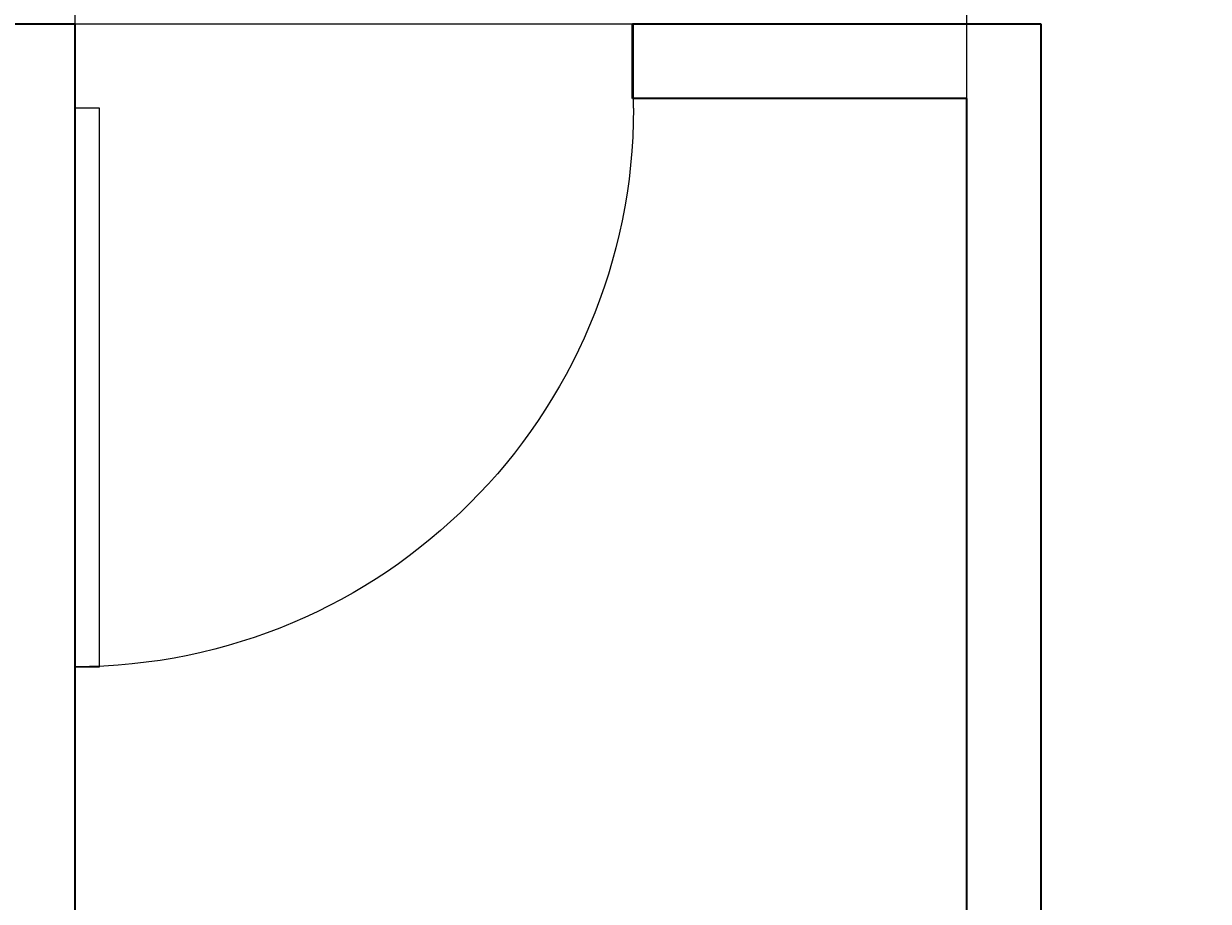
# Model space of a CAD drawing. Units: feet. Extents: x 105 to 1094, y -88 to 588.
# Tile 20 of 59: x 372 to 436, y 307 to 354. Entities that reach past the tile are written whole.
import ezdxf

# ---------------------------------------------------------------- set-up
doc = ezdxf.new("R2010")
doc.units = ezdxf.units.FT
doc.header["$MEASUREMENT"] = 0
for name, color, linetype, lineweight in [('A-ANNO-DIMS', 2, 'Continuous', 18), ('A-DOOR', 3, 'Continuous', 25), ('A-WALL', 7, 'Continuous', 35)]:
    doc.layers.add(name, color=color, linetype=linetype, lineweight=lineweight)
doc.styles.get("Standard").update_dxf_attribs({"font": 'arial.ttf'})
doc.dimstyles.get("Standard").update_dxf_attribs({"dimtxt": 0.18, "dimasz": 0.18, "dimexe": 0.18, "dimexo": 0.0625, "dimgap": 0.09, "dimtad": 0, "dimtih": 1, "dimtoh": 1, "dimdec": 4, "dimzin": 0, "dimdsep": 46, "dimtxsty": 'Standard', "dimcen": 0.09, "dimadec": 0, "dimazin": 0, "dimtfac": 1, "dimtdec": 4, "dimtofl": 0, "dimtmove": 0, "dimatfit": 3, "dimfxl": 1, "dimtolj": 1, "dimtzin": 0, "dimarcsym": 0})

# ---------------------------------------------------------------- blocks, each defined once
blk = doc.blocks.new('*U2')
for p, q in [((0, 0), (0, -6)), ((40, 0), (40, -6))]:
    blk.add_line(p, q)
blk.add_lwpolyline([(0, 0), (0, 40), (1.75, 40), (1.75, 0)], close=True)
blk.add_arc((0, 0), 40, 0, 90)
blk = doc.blocks.new('*D21')
at = {"layer": 'A-ANNO-DIMS', "color": 0, "lineweight": -2, "transparency": 16777216}
for p, q in [((849.626, 543.081), (105.458, 543.081)), ((105.638, 542.901), (105.638, 250.263)), ((105.638, -42.739), (105.638, 249.899)), ((849.626, -42.919), (105.458, -42.919))]:
    blk.add_line(p, q, dxfattribs=at)
at = {"layer": 'A-ANNO-DIMS', "color": 0, "transparency": 16777216}
for points in [[(105.608, 542.901), (105.668, 542.901), (105.638, 543.081)], [(105.608, -42.739), (105.668, -42.739), (105.638, -42.919)]]:
    blk.add_solid(points, dxfattribs=at)
at = {"layer": 'Defpoints', "color": 0, "transparency": 16777216}
for p in [(105.638, 543.081), (849.688, 543.081), (849.688, -42.919)]:
    blk.add_point(p, dxfattribs=at)
at = {"layer": 'A-ANNO-DIMS', "color": 0, "transparency": 16777216, "insert": (105.638, 250.081), "char_height": 0.18, "attachment_point": 5}
blk.add_mtext('\\A1;586', dxfattribs=at)
blk = doc.blocks.new('*D33')
at = {"layer": 'A-ANNO-DIMS', "color": 0, "lineweight": -2, "transparency": 16777216}
for p, q in [((646.626, 395.081), (105.458, 395.081)), ((105.638, 394.901), (105.638, 345.263)), ((105.638, 295.261), (105.638, 344.899)), ((646.626, 295.081), (105.458, 295.081))]:
    blk.add_line(p, q, dxfattribs=at)
at = {"layer": 'A-ANNO-DIMS', "color": 0, "transparency": 16777216}
for points in [[(105.608, 394.901), (105.668, 394.901), (105.638, 395.081)], [(105.608, 295.261), (105.668, 295.261), (105.638, 295.081)]]:
    blk.add_solid(points, dxfattribs=at)
at = {"layer": 'Defpoints', "color": 0, "transparency": 16777216}
for p in [(646.688, 395.081), (105.638, 295.081), (646.688, 295.081)]:
    blk.add_point(p, dxfattribs=at)
at = {"layer": 'A-ANNO-DIMS', "color": 0, "transparency": 16777216, "insert": (105.638, 345.081), "char_height": 0.18, "attachment_point": 5}
blk.add_mtext('\\A1;100', dxfattribs=at)
blk = doc.blocks.new('*D51')
at = {"layer": 'A-ANNO-DIMS', "color": 0, "lineweight": -2, "transparency": 16777216}
for p, q in [((432.626, 394.081), (105.458, 394.081)), ((105.638, 393.901), (105.638, 374.263)), ((105.638, 354.261), (105.638, 373.899)), ((426.626, 354.081), (105.458, 354.081))]:
    blk.add_line(p, q, dxfattribs=at)
at = {"layer": 'A-ANNO-DIMS', "color": 0, "transparency": 16777216}
for points in [[(105.608, 393.901), (105.668, 393.901), (105.638, 394.081)], [(105.608, 354.261), (105.668, 354.261), (105.638, 354.081)]]:
    blk.add_solid(points, dxfattribs=at)
at = {"layer": 'Defpoints', "color": 0, "transparency": 16777216}
for p in [(432.688, 394.081), (105.638, 354.081), (426.688, 354.081)]:
    blk.add_point(p, dxfattribs=at)
at = {"layer": 'A-ANNO-DIMS', "color": 0, "transparency": 16777216, "insert": (105.638, 374.081), "char_height": 0.18, "attachment_point": 5}
blk.add_mtext('\\A1;40', dxfattribs=at)
blk = doc.blocks.new('*D56')
at = {"layer": 'A-ANNO-DIMS', "color": 0, "lineweight": -2, "transparency": 16777216}
for p, q in [((374.688, 252.144), (374.688, 588.311)), ((374.868, 588.131), (398.466, 588.131)), ((422.508, 588.131), (398.911, 588.131)), ((422.688, 252.144), (422.688, 588.311))]:
    blk.add_line(p, q, dxfattribs=at)
at = {"layer": 'A-ANNO-DIMS', "color": 0, "transparency": 16777216}
for points in [[(374.868, 588.161), (374.868, 588.101), (374.688, 588.131)], [(422.508, 588.161), (422.508, 588.101), (422.688, 588.131)]]:
    blk.add_solid(points, dxfattribs=at)
at = {"layer": 'Defpoints', "color": 0, "transparency": 16777216}
for p in [(422.688, 588.131), (374.688, 252.081), (422.688, 252.081)]:
    blk.add_point(p, dxfattribs=at)
at = {"layer": 'A-ANNO-DIMS', "color": 0, "transparency": 16777216, "insert": (398.688, 588.131), "char_height": 0.18, "attachment_point": 5}
blk.add_mtext('\\A1;48', dxfattribs=at)

msp = doc.modelspace()

# ---------------------------------------------------------------- linework, layer by layer
at = {"layer": 'A-WALL'}
for p, q in [((374.6883, 354.0812), (288.6883, 354.0812)), ((374.6883, 252.0812), (374.6883, 354.0812)), ((426.6883, 354.0812), (404.6883, 354.0812)), ((404.6883, 350.0812), (404.6883, 354.0812)), ((426.6883, 252.0812), (426.6883, 354.0812)), ((422.6883, 350.0812), (404.6883, 350.0812)), ((422.6883, 252.0812), (422.6883, 350.0812))]:
    msp.add_line(p, q, dxfattribs=at)

# ---------------------------------------------------------------- block references
at = {"layer": 'A-DOOR', "xscale": -0.7513941790917756, "yscale": 0.7513941790917756, "zscale": 0.7513941790917756, "rotation": 180}
msp.add_blockref('*U2', (374.6883, 349.5728), dxfattribs=at)

# ---------------------------------------------------------------- dimensions: what is measured, and where the dimension line sits
at = {"layer": 'A-ANNO-DIMS'}
dim = msp.add_linear_dim(base=(422.6883, 588.1312), p1=(374.6883, 252.0812), p2=(422.6883, 252.0812), dimstyle='Standard', override={"dimdec": 0, "dimlfac": 1, "dimrnd": 0, "dimzin": 0, "dimdsep": 46, "dimlunit": 2}, dxfattribs=at)
dim.commit()
dim.dimension.update_dxf_attribs({"geometry": '*D56', "text_midpoint": (398.6883, 588.1312)})
for base, p1, p2, picture, middle in [((105.6383, 543.0812), (849.6883, -42.9188), (849.6883, 543.0812), '*D21', (105.6383, 250.0812)), ((105.6383, 295.0812), (646.6883, 395.0812), (646.6883, 295.0812), '*D33', (105.6383, 345.0812)), ((105.6383, 354.0812), (432.6883, 394.0812), (426.6883, 354.0812), '*D51', (105.6383, 374.0812))]:
    dim = msp.add_linear_dim(base=base, p1=p1, p2=p2, angle=90, dimstyle='Standard', override={"dimdec": 0, "dimlfac": 1, "dimrnd": 0, "dimzin": 0, "dimdsep": 46, "dimlunit": 2}, dxfattribs=at)
    dim.commit()
    dim.dimension.update_dxf_attribs({"geometry": picture, "text_midpoint": middle})

doc.saveas('drawing.dxf')
